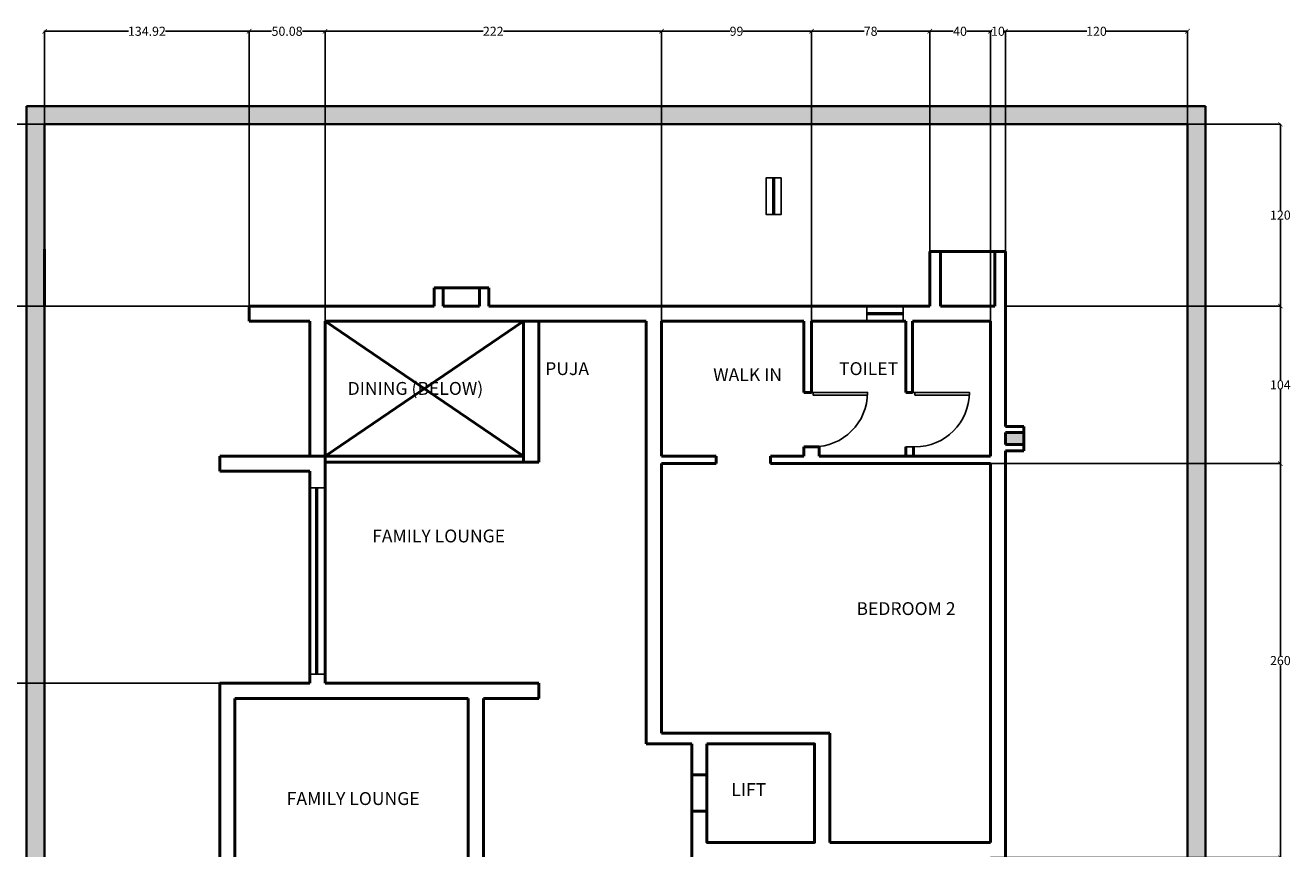
# Model space of a CAD drawing. Units: inches. Extents: x 925 to 2834, y 111 to 1355.
# Tile 25 of 25: x 1996 to 2831, y 699 to 1243. Entities that reach past the tile are written whole.
import ezdxf

# ---------------------------------------------------------------- set-up
doc = ezdxf.new("R2010")
doc.units = ezdxf.units.IN
doc.header["$MEASUREMENT"] = 0
for name, color, linetype, lineweight in [('A-ANNO-DIMS', 2, 'Continuous', 18), ('A-ANNO-TTLB', 7, 'Continuous', 35), ('A-AREA-IDEN', 7, 'Continuous', 18), ('A-DOOR', 2, 'Continuous', 25), ('A-FLOR-PATT', 252, 'Continuous', 13), ('A-GLAZ', 3, 'Continuous', 25), ('A-WALL', 7, 'Continuous', 50), ('A-WALL-PATT', 8, 'Continuous', 13)]:
    doc.layers.add(name, color=color, linetype=linetype, lineweight=lineweight)
doc.styles.get("Standard").update_dxf_attribs({"font": 'arial.ttf'})
doc.dimstyles.get("Standard").update_dxf_attribs({"dimtxt": 6, "dimasz": 3, "dimexe": 0.18, "dimexo": 0.0625, "dimgap": 0.09, "dimtad": 0, "dimtih": 1, "dimtoh": 1, "dimdec": 1, "dimzin": 0, "dimdsep": 46, "dimlunit": 3, "dimtxsty": 'Standard', "dimblk": 'ARCHTICK', "dimcen": 0.09, "dimadec": 0, "dimazin": 0, "dimtfac": 1, "dimtdec": 1, "dimtofl": 0, "dimtmove": 0, "dimatfit": 3, "dimfxl": 1, "dimtolj": 1, "dimtzin": 0, "dimarcsym": 0})

# ---------------------------------------------------------------- blocks, each defined once
blk = doc.blocks.new('*U7')
for p, q in [((0, 0), (0, -6)), ((36, 0), (36, -6))]:
    blk.add_line(p, q)
blk.add_lwpolyline([(0, 0), (0, 36), (1.75, 36), (1.75, 0)], close=True)
blk.add_arc((0, 0), 36, 0, 90)
blk = doc.blocks.new('_ArchTick')
at = {"color": 0, "linetype": 'ByBlock', "const_width": 0.15}
blk.add_lwpolyline([(-0.5, -0.5), (0.5, 0.5)], dxfattribs=at)
blk = doc.blocks.new('*D54')
at = {"layer": 'A-ANNO-DIMS', "color": 0, "lineweight": -2, "transparency": 16777216}
for p, q in [((2008.76, 1177.46), (2008.76, 1238.93)), ((2008.76, 1238.75), (2063.99, 1238.75)), ((2143.68, 1238.75), (2088.45, 1238.75)), ((2143.68, 1057.46), (2143.68, 1238.93))]:
    blk.add_line(p, q, dxfattribs=at)
at = {"layer": 'Defpoints', "color": 0, "transparency": 16777216}
for p in [(2143.68, 1238.75), (2008.76, 1177.4), (2143.68, 1057.4)]:
    blk.add_point(p, dxfattribs=at)
at = {"layer": 'A-ANNO-DIMS', "color": 0, "lineweight": -2, "transparency": 16777216, "xscale": 3, "yscale": 3, "zscale": 3, "rotation": 180}
blk.add_blockref('_ArchTick', (2008.76, 1238.75), dxfattribs=at)
at = {"layer": 'A-ANNO-DIMS', "color": 0, "lineweight": -2, "transparency": 16777216, "xscale": 3, "yscale": 3, "zscale": 3}
blk.add_blockref('_ArchTick', (2143.68, 1238.75), dxfattribs=at)
at = {"layer": 'A-ANNO-DIMS', "color": 0, "transparency": 16777216, "insert": (2076.22, 1238.75), "char_height": 6, "attachment_point": 5}
blk.add_mtext('\\A1;134.92', dxfattribs=at)
blk = doc.blocks.new('*D55')
at = {"layer": 'A-ANNO-DIMS', "color": 0, "lineweight": -2, "transparency": 16777216}
for p, q in [((2143.68, 1057.46), (2143.68, 1238.93)), ((2143.68, 1238.75), (2158.5, 1238.75)), ((2193.76, 1238.75), (2178.94, 1238.75)), ((2193.76, 1047.46), (2193.76, 1238.93))]:
    blk.add_line(p, q, dxfattribs=at)
at = {"layer": 'Defpoints', "color": 0, "transparency": 16777216}
for p in [(2193.76, 1238.75), (2143.68, 1057.4), (2193.76, 1047.4)]:
    blk.add_point(p, dxfattribs=at)
at = {"layer": 'A-ANNO-DIMS', "color": 0, "lineweight": -2, "transparency": 16777216, "xscale": 3, "yscale": 3, "zscale": 3, "rotation": 180}
blk.add_blockref('_ArchTick', (2143.68, 1238.75), dxfattribs=at)
at = {"layer": 'A-ANNO-DIMS', "color": 0, "lineweight": -2, "transparency": 16777216, "xscale": 3, "yscale": 3, "zscale": 3}
blk.add_blockref('_ArchTick', (2193.76, 1238.75), dxfattribs=at)
at = {"layer": 'A-ANNO-DIMS', "color": 0, "transparency": 16777216, "insert": (2168.72, 1238.75), "char_height": 6, "attachment_point": 5}
blk.add_mtext('\\A1;50.08', dxfattribs=at)
blk = doc.blocks.new('*D56')
at = {"layer": 'A-ANNO-DIMS', "color": 0, "lineweight": -2, "transparency": 16777216}
for p, q in [((2193.76, 1047.46), (2193.76, 1238.93)), ((2193.76, 1238.75), (2298.02, 1238.75)), ((2415.76, 1238.75), (2311.5, 1238.75)), ((2415.76, 1047.46), (2415.76, 1238.93))]:
    blk.add_line(p, q, dxfattribs=at)
at = {"layer": 'Defpoints', "color": 0, "transparency": 16777216}
for p in [(2415.76, 1238.75), (2193.76, 1047.4), (2415.76, 1047.4)]:
    blk.add_point(p, dxfattribs=at)
at = {"layer": 'A-ANNO-DIMS', "color": 0, "lineweight": -2, "transparency": 16777216, "xscale": 3, "yscale": 3, "zscale": 3, "rotation": 180}
blk.add_blockref('_ArchTick', (2193.76, 1238.75), dxfattribs=at)
at = {"layer": 'A-ANNO-DIMS', "color": 0, "lineweight": -2, "transparency": 16777216, "xscale": 3, "yscale": 3, "zscale": 3}
blk.add_blockref('_ArchTick', (2415.76, 1238.75), dxfattribs=at)
at = {"layer": 'A-ANNO-DIMS', "color": 0, "transparency": 16777216, "insert": (2304.76, 1238.75), "char_height": 6, "attachment_point": 5}
blk.add_mtext('\\A1;222', dxfattribs=at)
blk = doc.blocks.new('*D57')
at = {"layer": 'A-ANNO-DIMS', "color": 0, "lineweight": -2, "transparency": 16777216}
for p, q in [((2415.76, 1047.46), (2415.76, 1238.93)), ((2415.76, 1238.75), (2460.86, 1238.75)), ((2514.76, 1238.75), (2469.65, 1238.75)), ((2514.76, 1047.46), (2514.76, 1238.93))]:
    blk.add_line(p, q, dxfattribs=at)
at = {"layer": 'Defpoints', "color": 0, "transparency": 16777216}
for p in [(2514.76, 1238.75), (2415.76, 1047.4), (2514.76, 1047.4)]:
    blk.add_point(p, dxfattribs=at)
at = {"layer": 'A-ANNO-DIMS', "color": 0, "lineweight": -2, "transparency": 16777216, "xscale": 3, "yscale": 3, "zscale": 3, "rotation": 180}
blk.add_blockref('_ArchTick', (2415.76, 1238.75), dxfattribs=at)
at = {"layer": 'A-ANNO-DIMS', "color": 0, "lineweight": -2, "transparency": 16777216, "xscale": 3, "yscale": 3, "zscale": 3}
blk.add_blockref('_ArchTick', (2514.76, 1238.75), dxfattribs=at)
at = {"layer": 'A-ANNO-DIMS', "color": 0, "transparency": 16777216, "insert": (2465.26, 1238.75), "char_height": 6, "attachment_point": 5}
blk.add_mtext('\\A1;99', dxfattribs=at)
blk = doc.blocks.new('*D58')
at = {"layer": 'A-ANNO-DIMS', "color": 0, "lineweight": -2, "transparency": 16777216}
for p, q in [((2514.76, 1047.46), (2514.76, 1238.93)), ((2514.76, 1238.75), (2549.39, 1238.75)), ((2592.76, 1238.75), (2558.13, 1238.75)), ((2592.76, 1057.46), (2592.76, 1238.93))]:
    blk.add_line(p, q, dxfattribs=at)
at = {"layer": 'Defpoints', "color": 0, "transparency": 16777216}
for p in [(2592.76, 1238.75), (2592.76, 1057.4), (2514.76, 1047.4)]:
    blk.add_point(p, dxfattribs=at)
at = {"layer": 'A-ANNO-DIMS', "color": 0, "lineweight": -2, "transparency": 16777216, "xscale": 3, "yscale": 3, "zscale": 3, "rotation": 180}
blk.add_blockref('_ArchTick', (2514.76, 1238.75), dxfattribs=at)
at = {"layer": 'A-ANNO-DIMS', "color": 0, "lineweight": -2, "transparency": 16777216, "xscale": 3, "yscale": 3, "zscale": 3}
blk.add_blockref('_ArchTick', (2592.76, 1238.75), dxfattribs=at)
at = {"layer": 'A-ANNO-DIMS', "color": 0, "transparency": 16777216, "insert": (2553.76, 1238.75), "char_height": 6, "attachment_point": 5}
blk.add_mtext('\\A1;78', dxfattribs=at)
blk = doc.blocks.new('*D59')
at = {"layer": 'A-ANNO-DIMS', "color": 0, "lineweight": -2, "transparency": 16777216}
for p, q in [((2592.76, 1057.46), (2592.76, 1238.93)), ((2592.76, 1238.75), (2608.26, 1238.75)), ((2632.76, 1238.75), (2617.26, 1238.75)), ((2632.76, 1047.46), (2632.76, 1238.93))]:
    blk.add_line(p, q, dxfattribs=at)
at = {"layer": 'Defpoints', "color": 0, "transparency": 16777216}
for p in [(2632.76, 1238.75), (2592.76, 1057.4), (2632.76, 1047.4)]:
    blk.add_point(p, dxfattribs=at)
at = {"layer": 'A-ANNO-DIMS', "color": 0, "lineweight": -2, "transparency": 16777216, "xscale": 3, "yscale": 3, "zscale": 3, "rotation": 180}
blk.add_blockref('_ArchTick', (2592.76, 1238.75), dxfattribs=at)
at = {"layer": 'A-ANNO-DIMS', "color": 0, "lineweight": -2, "transparency": 16777216, "xscale": 3, "yscale": 3, "zscale": 3}
blk.add_blockref('_ArchTick', (2632.76, 1238.75), dxfattribs=at)
at = {"layer": 'A-ANNO-DIMS', "color": 0, "transparency": 16777216, "insert": (2612.76, 1238.75), "char_height": 6, "attachment_point": 5}
blk.add_mtext('\\A1;40', dxfattribs=at)
blk = doc.blocks.new('*D60')
at = {"layer": 'A-ANNO-DIMS', "color": 0, "lineweight": -2, "transparency": 16777216}
for p, q in [((2632.76, 1047.46), (2632.76, 1238.93)), ((2632.76, 1238.75), (2633.66, 1238.75)), ((2642.76, 1238.75), (2641.85, 1238.75)), ((2642.76, 1057.46), (2642.76, 1238.93))]:
    blk.add_line(p, q, dxfattribs=at)
at = {"layer": 'Defpoints', "color": 0, "transparency": 16777216}
for p in [(2642.76, 1238.75), (2642.76, 1057.4), (2632.76, 1047.4)]:
    blk.add_point(p, dxfattribs=at)
at = {"layer": 'A-ANNO-DIMS', "color": 0, "lineweight": -2, "transparency": 16777216, "xscale": 3, "yscale": 3, "zscale": 3, "rotation": 180}
blk.add_blockref('_ArchTick', (2632.76, 1238.75), dxfattribs=at)
at = {"layer": 'A-ANNO-DIMS', "color": 0, "lineweight": -2, "transparency": 16777216, "xscale": 3, "yscale": 3, "zscale": 3}
blk.add_blockref('_ArchTick', (2642.76, 1238.75), dxfattribs=at)
at = {"layer": 'A-ANNO-DIMS', "color": 0, "transparency": 16777216, "insert": (2637.76, 1238.75), "char_height": 6, "attachment_point": 5}
blk.add_mtext('\\A1;10', dxfattribs=at)
blk = doc.blocks.new('*D61')
at = {"layer": 'A-ANNO-DIMS', "color": 0, "lineweight": -2, "transparency": 16777216}
for p, q in [((2642.76, 1057.46), (2642.76, 1238.93)), ((2642.76, 1238.75), (2696.33, 1238.75)), ((2762.76, 1238.75), (2709.18, 1238.75)), ((2762.76, 1177.46), (2762.76, 1238.93))]:
    blk.add_line(p, q, dxfattribs=at)
at = {"layer": 'Defpoints', "color": 0, "transparency": 16777216}
for p in [(2762.76, 1238.75), (2762.76, 1177.4), (2642.76, 1057.4)]:
    blk.add_point(p, dxfattribs=at)
at = {"layer": 'A-ANNO-DIMS', "color": 0, "lineweight": -2, "transparency": 16777216, "xscale": 3, "yscale": 3, "zscale": 3, "rotation": 180}
blk.add_blockref('_ArchTick', (2642.76, 1238.75), dxfattribs=at)
at = {"layer": 'A-ANNO-DIMS', "color": 0, "lineweight": -2, "transparency": 16777216, "xscale": 3, "yscale": 3, "zscale": 3}
blk.add_blockref('_ArchTick', (2762.76, 1238.75), dxfattribs=at)
at = {"layer": 'A-ANNO-DIMS', "color": 0, "transparency": 16777216, "insert": (2702.76, 1238.75), "char_height": 6, "attachment_point": 5}
blk.add_mtext('\\A1;120', dxfattribs=at)
blk = doc.blocks.new('*D72')
at = {"layer": 'A-ANNO-DIMS', "color": 0, "lineweight": -2, "transparency": 16777216}
for p, q in [((2632.82, 953.4), (2824.29, 953.4)), ((2824.11, 953.4), (2824.11, 826.55)), ((2824.11, 693.4), (2824.11, 820.24)), ((2632.82, 693.4), (2824.29, 693.4))]:
    blk.add_line(p, q, dxfattribs=at)
at = {"layer": 'Defpoints', "color": 0, "transparency": 16777216}
for p in [(2632.76, 953.4), (2824.11, 953.4), (2632.76, 693.4)]:
    blk.add_point(p, dxfattribs=at)
at = {"layer": 'A-ANNO-DIMS', "color": 0, "lineweight": -2, "transparency": 16777216, "xscale": 3, "yscale": 3, "zscale": 3}
for p, rotation in [((2824.11, 953.4), 90), ((2824.11, 693.4), 270)]:
    blk.add_blockref('_ArchTick', p, dxfattribs=dict(at, rotation=rotation))
at = {"layer": 'A-ANNO-DIMS', "color": 0, "transparency": 16777216, "insert": (2824.11, 823.4), "char_height": 6, "attachment_point": 5}
blk.add_mtext('\\A1;260', dxfattribs=at)
blk = doc.blocks.new('*D73')
at = {"layer": 'A-ANNO-DIMS', "color": 0, "lineweight": -2, "transparency": 16777216}
for p, q in [((2642.82, 1057.4), (2824.29, 1057.4)), ((2824.11, 1057.4), (2824.11, 1008.55)), ((2824.11, 953.4), (2824.11, 1002.24)), ((2632.82, 953.4), (2824.29, 953.4))]:
    blk.add_line(p, q, dxfattribs=at)
at = {"layer": 'Defpoints', "color": 0, "transparency": 16777216}
for p in [(2642.76, 1057.4), (2824.11, 1057.4), (2632.76, 953.4)]:
    blk.add_point(p, dxfattribs=at)
at = {"layer": 'A-ANNO-DIMS', "color": 0, "lineweight": -2, "transparency": 16777216, "xscale": 3, "yscale": 3, "zscale": 3}
for p, rotation in [((2824.11, 1057.4), 90), ((2824.11, 953.4), 270)]:
    blk.add_blockref('_ArchTick', p, dxfattribs=dict(at, rotation=rotation))
at = {"layer": 'A-ANNO-DIMS', "color": 0, "transparency": 16777216, "insert": (2824.11, 1005.4), "char_height": 6, "attachment_point": 5}
blk.add_mtext('\\A1;104', dxfattribs=at)
blk = doc.blocks.new('*D74')
at = {"layer": 'A-ANNO-DIMS', "color": 0, "lineweight": -2, "transparency": 16777216}
for p, q in [((2762.82, 1177.4), (2824.29, 1177.4)), ((2824.11, 1177.4), (2824.11, 1120.55)), ((2824.11, 1057.4), (2824.11, 1114.24)), ((2642.82, 1057.4), (2824.29, 1057.4))]:
    blk.add_line(p, q, dxfattribs=at)
at = {"layer": 'Defpoints', "color": 0, "transparency": 16777216}
for p in [(2762.76, 1177.4), (2824.11, 1177.4), (2642.76, 1057.4)]:
    blk.add_point(p, dxfattribs=at)
at = {"layer": 'A-ANNO-DIMS', "color": 0, "lineweight": -2, "transparency": 16777216, "xscale": 3, "yscale": 3, "zscale": 3}
for p, rotation in [((2824.11, 1177.4), 90), ((2824.11, 1057.4), 270)]:
    blk.add_blockref('_ArchTick', p, dxfattribs=dict(at, rotation=rotation))
at = {"layer": 'A-ANNO-DIMS', "color": 0, "transparency": 16777216, "insert": (2824.11, 1117.4), "char_height": 6, "attachment_point": 5}
blk.add_mtext('\\A1;120', dxfattribs=at)
blk = doc.blocks.new('*D78')
at = {"layer": 'A-ANNO-DIMS', "color": 0, "lineweight": -2, "transparency": 16777216}
for p, q in [((2124.2, 808.4), (1947.23, 808.4)), ((1947.41, 808.4), (1947.41, 723.55)), ((1947.41, 632.4), (1947.41, 717.24)), ((2134.2, 632.4), (1947.23, 632.4))]:
    blk.add_line(p, q, dxfattribs=at)
at = {"layer": 'Defpoints', "color": 0, "transparency": 16777216}
for p in [(1947.41, 808.4), (2124.26, 808.4), (2134.26, 632.4)]:
    blk.add_point(p, dxfattribs=at)
at = {"layer": 'A-ANNO-DIMS', "color": 0, "lineweight": -2, "transparency": 16777216, "xscale": 3, "yscale": 3, "zscale": 3}
for p, rotation in [((1947.41, 808.4), 90), ((1947.41, 632.4), 270)]:
    blk.add_blockref('_ArchTick', p, dxfattribs=dict(at, rotation=rotation))
at = {"layer": 'A-ANNO-DIMS', "color": 0, "transparency": 16777216, "insert": (1947.41, 720.4), "char_height": 6, "attachment_point": 5}
blk.add_mtext('\\A1;176', dxfattribs=at)
blk = doc.blocks.new('*D79')
at = {"layer": 'A-ANNO-DIMS', "color": 0, "lineweight": -2, "transparency": 16777216}
for p, q in [((2143.61, 1057.4), (1947.23, 1057.4)), ((1947.41, 1057.4), (1947.41, 936.05)), ((1947.41, 808.4), (1947.41, 929.74)), ((2124.2, 808.4), (1947.23, 808.4))]:
    blk.add_line(p, q, dxfattribs=at)
at = {"layer": 'Defpoints', "color": 0, "transparency": 16777216}
for p in [(1947.41, 1057.4), (2143.68, 1057.4), (2124.26, 808.4)]:
    blk.add_point(p, dxfattribs=at)
at = {"layer": 'A-ANNO-DIMS', "color": 0, "lineweight": -2, "transparency": 16777216, "xscale": 3, "yscale": 3, "zscale": 3}
for p, rotation in [((1947.41, 1057.4), 90), ((1947.41, 808.4), 270)]:
    blk.add_blockref('_ArchTick', p, dxfattribs=dict(at, rotation=rotation))
at = {"layer": 'A-ANNO-DIMS', "color": 0, "transparency": 16777216, "insert": (1947.41, 932.9), "char_height": 6, "attachment_point": 5}
blk.add_mtext('\\A1;249', dxfattribs=at)
blk = doc.blocks.new('*D80')
at = {"layer": 'A-ANNO-DIMS', "color": 0, "lineweight": -2, "transparency": 16777216}
for p, q in [((2008.7, 1177.4), (1947.23, 1177.4)), ((1947.41, 1177.4), (1947.41, 1120.55)), ((1947.41, 1057.4), (1947.41, 1114.24)), ((2143.61, 1057.4), (1947.23, 1057.4))]:
    blk.add_line(p, q, dxfattribs=at)
at = {"layer": 'Defpoints', "color": 0, "transparency": 16777216}
for p in [(1947.41, 1177.4), (2008.76, 1177.4), (2143.68, 1057.4)]:
    blk.add_point(p, dxfattribs=at)
at = {"layer": 'A-ANNO-DIMS', "color": 0, "lineweight": -2, "transparency": 16777216, "xscale": 3, "yscale": 3, "zscale": 3}
for p, rotation in [((1947.41, 1177.4), 90), ((1947.41, 1057.4), 270)]:
    blk.add_blockref('_ArchTick', p, dxfattribs=dict(at, rotation=rotation))
at = {"layer": 'A-ANNO-DIMS', "color": 0, "transparency": 16777216, "insert": (1947.41, 1117.4), "char_height": 6, "attachment_point": 5}
blk.add_mtext('\\A1;120', dxfattribs=at)

msp = doc.modelspace()

# ---------------------------------------------------------------- hatches: boundary and pattern name
at = {"layer": 'A-FLOR-PATT'}
h = msp.add_hatch(color=256, dxfattribs=at)
h.dxf.hatch_style = 1
h.paths.add_polyline_path([(2774.758, 1189.3964), (1996.758, 1189.3964), (1996.758, 228.8964), (2774.758, 228.8964)])
h.paths.add_polyline_path([(2008.758, 1177.3964), (2762.758, 1177.3964), (2762.758, 240.8964), (2008.758, 240.8964)], flags=16)
h.paths.add_polyline_path([(2107.276, 551.9993), (2124.258, 551.9993), (2124.258, 703.3964), (2134.258, 703.3964), (2158.258, 703.3964), (2183.758, 703.3964), (2183.758, 751.3964), (2183.758, 775.3964), (2183.758, 823.3964), (2183.758, 969.395), (2183.758, 1041.395), (2183.758, 1047.3964), (2143.677, 1047.3964), (2143.677, 1057.3964), (2217.758, 1057.3964), (2265.758, 1057.3964), (2265.758, 1069.3964), (2271.758, 1069.3964), (2271.758, 1057.3964), (2295.758, 1057.3964), (2295.758, 1069.3964), (2301.758, 1069.3964), (2301.758, 1057.3964), (2592.758, 1057.3964), (2592.758, 1093.3964), (2599.758, 1093.3964), (2599.758, 1057.3964), (2635.758, 1057.3964), (2635.758, 1093.3964), (2642.758, 1093.3964), (2642.758, 1057.3964), (2642.758, 1025.9327), (2639.758, 1025.9327), (2639.758, 1001.9327), (2639.758, 977.9327), (2642.758, 977.9327), (2654.758, 977.9327), (2654.758, 973.9327), (2654.758, 965.9327), (2654.758, 961.9327), (2642.758, 961.9327), (2642.758, 869.3964), (2639.4187, 869.3964), (2639.4187, 867.3964), (2637.4187, 867.3964, 0.41421356), (2601.4187, 831.3964), (2637.4187, 831.3964), (2637.4187, 829.3964), (2639.4187, 829.3964), (2639.4187, 827.3964), (2642.758, 827.3964), (2642.758, 797.3943), (2658.5108, 797.3943), (2658.4187, 795.3964, -0.41421356), (2636.4868, 769.3964), (2636.4868, 767.3964), (2642.758, 767.3964), (2642.758, 693.3964), (2642.758, 645.3964), (2656.758, 645.3964), (2656.758, 641.3964), (2656.758, 617.3964), (2656.758, 610.3964), (2656.758, 586.3964), (2656.758, 579.3964), (2642.758, 579.3964), (2642.758, 360.8964), (2358.258, 360.8964), (2358.258, 408.8964), (2358.258, 506.3964), (2334.258, 506.3964), (2332.258, 506.3964), (2332.258, 508.3964, 0.41421356), (2296.258, 544.3964), (2296.258, 508.3964), (2294.258, 508.3964), (2294.258, 506.3964), (2292.258, 506.3964), (2206.258, 506.3964), (2134.258, 506.3964), (2124.258, 506.3964), (2124.258, 517.9993), (2107.276, 517.9993), (2107.276, 521.9993), (2124.258, 521.9993), (2124.258, 547.9993), (2107.276, 547.9993)], flags=0)
h.paths.add_polyline_path([(2134.258, 693.3964), (2134.258, 698.8964), (2158.258, 698.8964), (2158.258, 693.3964), (2368.258, 693.3964), (2368.258, 703.3964), (2193.758, 703.3964), (2188.258, 703.3964), (2188.258, 751.3964), (2193.758, 751.3964), (2193.758, 775.3964), (2188.258, 775.3964), (2188.258, 823.3964), (2193.758, 823.3964), (2193.758, 869.3964), (2193.758, 879.3964), (2193.758, 969.395), (2188.758, 969.395), (2188.758, 1005.395), (2189.758, 1005.395), (2189.758, 1041.395), (2193.758, 1041.395), (2193.758, 1047.3964), (2217.758, 1047.3964), (2217.758, 1052.8964), (2265.758, 1052.8964), (2265.758, 1051.8964), (2217.758, 1051.8964), (2217.758, 1047.3964), (2193.758, 1047.3964), (2193.758, 1041.395), (2190.758, 1041.395), (2190.758, 1005.395), (2189.758, 1005.395), (2189.758, 969.395), (2193.758, 969.395), (2193.758, 879.3964), (2193.758, 869.3964), (2193.758, 823.3964), (2189.258, 823.3964), (2189.258, 775.3964), (2193.758, 775.3964), (2193.758, 751.3964), (2189.258, 751.3964), (2189.258, 703.3964), (2193.758, 703.3964), (2368.258, 703.3964), (2368.258, 693.3964), (2158.258, 693.3964), (2158.258, 697.8964), (2134.258, 697.8964), (2134.258, 693.3964), (2134.258, 516.3964), (2134.258, 511.8964), (2206.258, 511.8964), (2206.258, 510.8964), (2134.258, 510.8964), (2134.258, 516.3964)], flags=0)
h.paths.add_polyline_path([(2374.258, 610.7178), (2376.258, 610.7178), (2376.258, 645.3964), (2378.258, 645.3964, -0.40021217), (2414.2165, 611.1251), (2416.258, 611.1251), (2416.258, 617.3964), (2488.758, 617.3964), (2488.758, 653.3964), (2596.758, 653.3964), (2596.758, 657.3964), (2488.758, 657.3964), (2488.758, 693.3964), (2435.758, 693.3964), (2435.758, 723.8964), (2435.758, 747.8964), (2435.758, 775.3964), (2435.758, 833.3964), (2435.9366, 833.3964), (2435.9366, 835.3964), (2439.6653, 835.3964, 0.41421356), (2461.5973, 855.3964), (2437.5973, 855.3964), (2435.9366, 855.3964), (2435.9366, 857.3964), (2435.758, 857.3964), (2435.758, 869.3964), (2375.758, 869.3964), (2375.758, 879.3964), (2516.758, 879.3964), (2516.758, 914.3964), (2516.758, 916.3964), (2520.4868, 916.3964, 0.41421356), (2542.4187, 942.3964), (2518.4187, 942.3964), (2516.758, 942.3964), (2516.758, 944.3964), (2520.0795, 944.3964), (2526.758, 944.3964), (2632.758, 944.3964), (2632.758, 879.3964), (2526.758, 879.3964), (2526.758, 914.3964), (2516.758, 914.3964), (2516.758, 879.3964), (2375.758, 879.3964), (2375.758, 869.3964), (2435.758, 869.3964), (2435.758, 857.3964), (2442.758, 857.3964), (2442.758, 869.3964), (2516.758, 869.3964), (2516.758, 775.3964), (2442.758, 775.3964), (2442.758, 833.3964), (2435.758, 833.3964), (2435.758, 775.3964), (2435.758, 747.8964), (2445.758, 747.8964), (2445.758, 768.3964), (2516.758, 768.3964), (2516.758, 703.3964), (2445.758, 703.3964), (2445.758, 723.8964), (2435.758, 723.8964), (2435.758, 693.3964), (2632.758, 693.3964), (2638.258, 693.3964), (2638.258, 645.3964), (2632.758, 645.3964), (2632.758, 617.3964), (2416.258, 617.3964), (2416.258, 607.3964), (2545.258, 607.3964), (2545.258, 418.8964), (2549.758, 418.8964), (2549.758, 478.8964), (2549.758, 483.3964), (2549.758, 607.3964), (2632.758, 607.3964), (2632.758, 483.3964), (2579.758, 483.3964), (2579.758, 478.8964), (2632.758, 478.8964), (2632.758, 370.8964), (2549.758, 370.8964), (2549.758, 394.8964), (2545.258, 394.8964), (2545.258, 370.8964), (2406.258, 370.8964), (2406.258, 364.8964), (2362.258, 364.8964), (2362.258, 367.6686), (2362.258, 408.8964), (2368.258, 408.8964), (2368.258, 607.3964), (2374.258, 607.3964)], flags=0)
h.paths.add_polyline_path([(2368.258, 408.8964), (2368.258, 370.8964), (2406.258, 370.8964), (2406.258, 366.8964), (2364.258, 366.8964), (2364.258, 367.6686), (2364.258, 408.8964)], flags=0)
h.paths.add_polyline_path([(2229.758, 869.3964), (2229.758, 879.3964), (2301.758, 879.3964), (2301.758, 869.3964)], flags=0)
h.paths.add_polyline_path([(2488.758, 638.1212), (2489.8812, 639.6555), (2489.5021, 638.621), (2490.027, 638.1212), (2489.5021, 637.6214), (2489.8812, 636.5869)], flags=0)
h.paths.add_polyline_path([(2499.4891, 671.007), (2500.014, 671.5068), (2499.6349, 672.5413), (2500.758, 671.007), (2499.6349, 669.4727), (2500.014, 670.5072)], flags=0)
h.paths.add_polyline_path([(2632.758, 797.3964), (2636.0795, 797.3964), (2636.0795, 795.3964), (2634.4187, 795.3964), (2632.758, 795.3964)], flags=0)
at = {"layer": 'A-WALL-PATT', "transparency": 33554605}
h = msp.add_hatch(color=256, dxfattribs=at)
h.dxf.hatch_style = 1
h.paths.add_polyline_path([(2656.758, 610.3964), (2639.758, 610.3964), (2639.758, 586.3964), (2656.758, 586.3964)])
h.paths.add_polyline_path([(2656.758, 641.3964), (2639.758, 641.3964), (2639.758, 617.3964), (2656.758, 617.3964)])
h.paths.add_polyline_path([(2654.758, 973.9327), (2642.758, 973.9327), (2642.758, 965.9327), (2654.758, 965.9327)])

# ---------------------------------------------------------------- linework, layer by layer
at = {"layer": 'A-ANNO-TTLB'}
for p, q in [((2774.758, 1189.3964), (1996.758, 1189.3964)), ((1996.758, 1189.3964), (1996.758, 228.8964)), ((2774.758, 228.8964), (2774.758, 1189.3964)), ((2762.758, 1177.3964), (2008.758, 1177.3964)), ((2008.758, 1177.3964), (2008.758, 240.8964)), ((2642.758, 1177.3964), (2762.758, 1177.3964)), ((2762.758, 1177.3964), (2762.758, 240.8964)), ((2762.758, 240.8964), (2762.758, 1177.3964)), ((2762.758, 240.8964), (2762.758, 1057.3964))]:
    msp.add_line(p, q, dxfattribs=at)
at = {"layer": 'A-DOOR'}
for p, q in [((2187.758, 937.4505), (2187.758, 856.4622)), ((2188.758, 937.4505), (2188.758, 856.4622)), ((2187.758, 856.4622), (2188.758, 856.4622)), ((2187.758, 814.4622), (2187.758, 856.4622)), ((2187.758, 856.4622), (2188.758, 856.4622)), ((2188.758, 814.4622), (2188.758, 856.4622))]:
    msp.add_line(p, q, dxfattribs=at)
msp.add_lwpolyline([(2193.758, 937.4505), (2193.758, 814.4622), (2183.758, 814.4622), (2183.758, 937.4505)], close=True, dxfattribs=at)
at = {"layer": 'A-GLAZ'}
for p, q in [((2489.2835, 1141.9078), (2489.2835, 1117.9078)), ((2489.7835, 1141.9078), (2489.7835, 1117.9078)), ((2490.2835, 1141.9078), (2490.2835, 1117.9078)), ((2551.2821, 1052.8964), (2575.2821, 1052.8964)), ((2551.2821, 1052.3964), (2575.2821, 1052.3964)), ((2551.2821, 1051.8964), (2575.2821, 1051.8964))]:
    msp.add_line(p, q, dxfattribs=at)
for points in [[(2494.7835, 1141.9078), (2494.7835, 1117.9078), (2484.7835, 1117.9078), (2484.7835, 1141.9078)], [(2551.2821, 1057.3964), (2575.2821, 1057.3964), (2575.2821, 1047.3964), (2551.2821, 1047.3964)]]:
    msp.add_lwpolyline(points, close=True, dxfattribs=at)
at = {"layer": 'A-WALL'}
for p, q in [((2008.758, 1094.9228), (2008.758, 1057.3964)), ((2592.758, 1057.3964), (2592.758, 1093.3964)), ((2592.758, 1093.3964), (2599.758, 1093.3964)), ((2599.758, 1057.3964), (2599.758, 1093.3964)), ((2599.758, 1093.3964), (2635.758, 1093.3964)), ((2635.758, 1057.3964), (2635.758, 1093.3964)), ((2635.758, 1093.3964), (2642.758, 1093.3964)), ((2642.758, 1057.3964), (2642.758, 1093.3964)), ((2265.758, 1057.3964), (2265.758, 1069.3964)), ((2265.758, 1069.3964), (2271.758, 1069.3964)), ((2271.758, 1057.3964), (2271.758, 1069.3964)), ((2271.758, 1069.3964), (2295.758, 1069.3964)), ((2295.758, 1057.3964), (2295.758, 1069.3964)), ((2295.758, 1069.3964), (2301.758, 1069.3964)), ((2301.758, 1057.3964), (2301.758, 1069.3964)), ((2143.677, 1047.3964), (2143.677, 1057.3964)), ((2217.758, 1057.3964), (2143.677, 1057.3964)), ((2217.758, 1057.3964), (2265.758, 1057.3964)), ((2271.758, 1057.3964), (2295.758, 1057.3964)), ((2301.758, 1057.3964), (2592.758, 1057.3964)), ((2599.758, 1057.3964), (2635.758, 1057.3964)), ((2642.758, 1057.3964), (2642.758, 1025.9327)), ((2642.758, 1057.3964), (2642.758, 1025.9327)), ((2143.677, 1047.3964), (2183.758, 1047.3964)), ((2183.758, 1047.3964), (2183.758, 1041.395)), ((2183.758, 1047.3964), (2183.758, 958.3964)), ((2193.758, 1047.3964), (2193.758, 1041.395)), ((2193.758, 1047.3964), (2193.758, 879.3964)), ((2193.758, 1047.3964), (2217.758, 1047.3964)), ((2193.758, 958.3964), (2324.758, 1047.3964)), ((2193.758, 1047.3964), (2324.758, 958.3964)), ((2217.758, 1047.3964), (2265.758, 1047.3964)), ((2265.758, 1047.3964), (2405.758, 1047.3964)), ((2324.758, 958.3964), (2324.758, 1047.3964)), ((2334.758, 954.3964), (2334.758, 1047.3964)), ((2405.758, 958.3964), (2405.758, 1047.3964)), ((2415.758, 958.3964), (2415.758, 1047.3964)), ((2415.758, 1047.3964), (2509.758, 1047.3964)), ((2509.758, 1000.3964), (2509.758, 1047.3964)), ((2514.758, 1000.3964), (2514.758, 1047.3964)), ((2514.758, 1047.3964), (2576.952, 1047.3964)), ((2576.952, 1047.3964), (2576.952, 1000.3964)), ((2581.452, 1047.3964), (2581.452, 1000.3964)), ((2581.452, 1047.3964), (2632.758, 1047.3964)), ((2632.758, 958.3964), (2632.758, 1047.3964)), ((2642.758, 977.9327), (2642.758, 1025.9327)), ((2514.758, 1000.3964), (2509.758, 1000.3964)), ((2576.952, 1000.3964), (2581.452, 1000.3964)), ((2642.758, 977.9327), (2654.758, 977.9327)), ((2654.758, 973.9327), (2654.758, 977.9327)), ((2654.758, 977.9327), (2654.758, 961.9327)), ((2642.758, 973.9327), (2642.758, 965.9327)), ((2642.758, 973.9327), (2654.758, 973.9327)), ((2654.758, 965.9327), (2654.758, 973.9327)), ((2509.758, 964.3964), (2509.758, 958.3964)), ((2519.758, 964.3964), (2509.758, 964.3964)), ((2519.758, 964.3964), (2519.758, 958.3964)), ((2576.952, 958.3964), (2576.952, 964.3964)), ((2581.952, 958.3964), (2581.952, 964.3964)), ((2642.758, 965.9327), (2654.758, 965.9327)), ((2642.758, 961.9327), (2654.758, 961.9327)), ((2642.758, 869.3964), (2642.758, 961.9327)), ((2654.758, 961.9327), (2642.758, 961.9327)), ((2642.758, 961.9327), (2642.758, 869.3964)), ((2642.758, 645.3964), (2642.758, 961.9327)), ((2654.758, 961.9327), (2654.758, 965.9327)), ((2183.758, 958.3964), (2124.258, 958.3964)), ((2124.258, 958.3964), (2124.258, 948.3964)), ((2193.758, 958.3964), (2183.758, 958.3964)), ((2193.758, 958.3964), (2324.758, 958.3964)), ((2193.758, 954.3964), (2334.758, 954.3964)), ((2324.758, 958.3964), (2324.758, 954.3964)), ((2405.758, 958.3964), (2405.758, 768.3964)), ((2415.758, 958.3964), (2451.758, 958.3964)), ((2415.758, 953.3964), (2415.758, 775.3964)), ((2415.758, 953.3964), (2451.758, 953.3964)), ((2451.758, 953.3964), (2451.758, 958.3964)), ((2487.758, 953.3964), (2487.758, 958.3964)), ((2487.758, 958.3964), (2509.758, 958.3964)), ((2487.758, 953.3964), (2632.758, 953.3964)), ((2519.758, 958.3964), (2576.952, 958.3964)), ((2576.952, 958.3964), (2581.452, 958.3964)), ((2581.452, 958.3964), (2632.758, 958.3964)), ((2632.758, 953.3964), (2632.758, 703.3964)), ((2632.758, 953.3964), (2632.758, 869.3964)), ((2632.758, 953.3964), (2632.758, 951.3964)), ((2183.758, 948.3964), (2124.258, 948.3964)), ((2183.758, 948.3964), (2183.758, 808.3964)), ((2632.758, 944.3964), (2632.758, 938.3964)), ((2193.758, 869.3964), (2193.758, 879.3964)), ((2193.758, 869.3964), (2193.758, 808.3964)), ((2632.758, 827.3964), (2632.758, 804.3964)), ((2642.758, 827.3964), (2642.758, 797.3964)), ((2642.758, 827.3964), (2642.758, 797.3964)), ((2124.258, 808.3964), (2124.258, 551.9993)), ((2124.258, 808.3964), (2183.758, 808.3964)), ((2134.258, 808.3964), (2183.758, 808.3964)), ((2193.758, 808.3964), (2334.758, 808.3964)), ((2334.758, 808.3964), (2334.758, 798.3964)), ((2134.258, 798.3964), (2288.258, 798.3964)), ((2134.258, 637.3964), (2134.258, 798.3964)), ((2288.258, 637.3964), (2288.258, 798.3964)), ((2298.258, 632.3964), (2298.258, 798.3964)), ((2298.258, 798.3964), (2334.758, 798.3964)), ((2435.758, 768.3964), (2405.758, 768.3964)), ((2435.758, 775.3964), (2415.758, 775.3964)), ((2435.758, 775.3964), (2526.758, 775.3964)), ((2435.758, 768.3964), (2435.758, 747.8964)), ((2445.758, 768.3964), (2445.758, 747.8964)), ((2445.758, 768.3964), (2516.758, 768.3964)), ((2516.758, 768.3964), (2516.758, 703.3964)), ((2526.758, 775.3964), (2526.758, 703.3964)), ((2642.758, 767.3964), (2642.758, 693.3964)), ((2445.758, 747.8964), (2435.758, 747.8964)), ((2435.758, 723.8964), (2435.758, 747.8964)), ((2435.758, 723.8964), (2435.758, 693.3964)), ((2435.758, 723.8964), (2445.758, 723.8964)), ((2445.758, 723.8964), (2445.758, 703.3964)), ((2516.758, 703.3964), (2445.758, 703.3964)), ((2632.758, 703.3964), (2526.758, 703.3964)), ((2642.758, 703.3964), (2642.758, 693.3964))]:
    msp.add_line(p, q, dxfattribs=at)
msp.add_lwpolyline([(2445.758, 768.3964), (2516.758, 768.3964), (2516.758, 703.3964), (2445.758, 703.3964)], close=True, dxfattribs=at)

# ---------------------------------------------------------------- block references
at = {"layer": 'A-DOOR', "rotation": 270}
for p in [(2515.758, 1000.3964), (2582.952, 1000.3964)]:
    msp.add_blockref('*U7', p, dxfattribs=at)

# ---------------------------------------------------------------- texts
at = {"layer": 'A-AREA-IDEN'}
for s, height, p in [('PUJA ', 8.49473, (2339.0344, 1011.8334)), ('TOILET', 8.49473, (2532.9193, 1011.8334)), ('WALK IN', 8.49473, (2449.8894, 1007.8817)), ('DINING (BELOW)', 8.494735, (2208.6973, 998.772)), ('FAMILY LOUNGE', 8.494735, (2224.8366, 901.3954)), ('BEDROOM 2', 8.49473, (2544.4033, 853.4416)), ('FAMILY LOUNGE', 8.494735, (2168.4816, 728.0699)), ('LIFT', 8.49473, (2461.8494, 733.985))]:
    msp.add_text(s, height=height, dxfattribs=at).set_placement(p)

# ---------------------------------------------------------------- dimensions: what is measured, and where the dimension line sits
at = {"layer": 'A-ANNO-DIMS'}
for base, p1, p2, override, picture, middle in [((2143.677, 1238.7464), (2008.758, 1177.3964), (2143.677, 1057.3964), {"dimdec": 2, "dimlfac": 1, "dimrnd": 0, "dimzin": 0, "dimdsep": 46, "dimlunit": 2}, '*D54', (2076.2175, 1238.7464)), ((2193.758, 1238.7464), (2143.677, 1057.3964), (2193.758, 1047.3964), {"dimdec": 2, "dimlfac": 1, "dimrnd": 0, "dimzin": 0, "dimdsep": 46, "dimlunit": 2}, '*D55', (2168.7175, 1238.7464)), ((2415.758, 1238.7464), (2193.758, 1047.3964), (2415.758, 1047.3964), {"dimdec": 0, "dimlfac": 1, "dimrnd": 0, "dimzin": 0, "dimdsep": 46, "dimlunit": 2}, '*D56', (2304.758, 1238.7464)), ((2514.758, 1238.7464), (2415.758, 1047.3964), (2514.758, 1047.3964), {"dimdec": 0, "dimlfac": 1, "dimrnd": 0, "dimzin": 0, "dimdsep": 46, "dimlunit": 2}, '*D57', (2465.258, 1238.7464)), ((2592.758, 1238.7464), (2514.758, 1047.3964), (2592.758, 1057.3964), {"dimdec": 0, "dimlfac": 1, "dimrnd": 0, "dimzin": 0, "dimdsep": 46, "dimlunit": 2}, '*D58', (2553.758, 1238.7464)), ((2632.758, 1238.7464), (2592.758, 1057.3964), (2632.758, 1047.3964), {"dimdec": 0, "dimlfac": 1, "dimrnd": 0, "dimzin": 0, "dimdsep": 46, "dimlunit": 2}, '*D59', (2612.758, 1238.7464)), ((2642.758, 1238.7464), (2632.758, 1047.3964), (2642.758, 1057.3964), {"dimdec": 0, "dimlfac": 1, "dimrnd": 0, "dimzin": 0, "dimdsep": 46, "dimlunit": 2}, '*D60', (2637.758, 1238.7464)), ((2762.758, 1238.7464), (2642.758, 1057.3964), (2762.758, 1177.3964), {"dimdec": 0, "dimlfac": 1, "dimrnd": 0, "dimzin": 0, "dimdsep": 46, "dimlunit": 2}, '*D61', (2702.758, 1238.7464))]:
    dim = msp.add_linear_dim(base=base, p1=p1, p2=p2, dimstyle='Standard', override=override, dxfattribs=at)
    dim.commit()
    dim.dimension.update_dxf_attribs({"geometry": picture, "text_midpoint": middle})
for base, p1, p2, picture, middle in [((1947.408, 1177.3964), (2143.677, 1057.3964), (2008.758, 1177.3964), '*D80', (1947.408, 1117.3964)), ((2824.108, 1177.3964), (2642.758, 1057.3964), (2762.758, 1177.3964), '*D74', (2824.108, 1117.3964)), ((1947.408, 1057.3964), (2124.258, 808.3964), (2143.677, 1057.3964), '*D79', (1947.408, 932.8964)), ((2824.108, 1057.3964), (2632.758, 953.3964), (2642.758, 1057.3964), '*D73', (2824.108, 1005.3964)), ((2824.108, 953.3964), (2632.758, 693.3964), (2632.758, 953.3964), '*D72', (2824.108, 823.3964)), ((1947.408, 808.3964), (2134.258, 632.3964), (2124.258, 808.3964), '*D78', (1947.408, 720.3964))]:
    dim = msp.add_linear_dim(base=base, p1=p1, p2=p2, angle=90, dimstyle='Standard', override={"dimdec": 0, "dimlfac": 1, "dimrnd": 0, "dimzin": 0, "dimdsep": 46, "dimlunit": 2}, dxfattribs=at)
    dim.commit()
    dim.dimension.update_dxf_attribs({"geometry": picture, "text_midpoint": middle})

doc.saveas('drawing.dxf')
